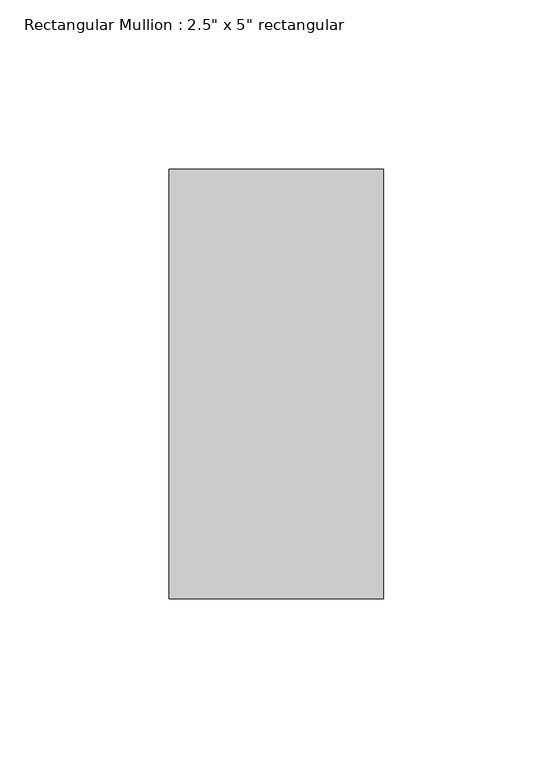
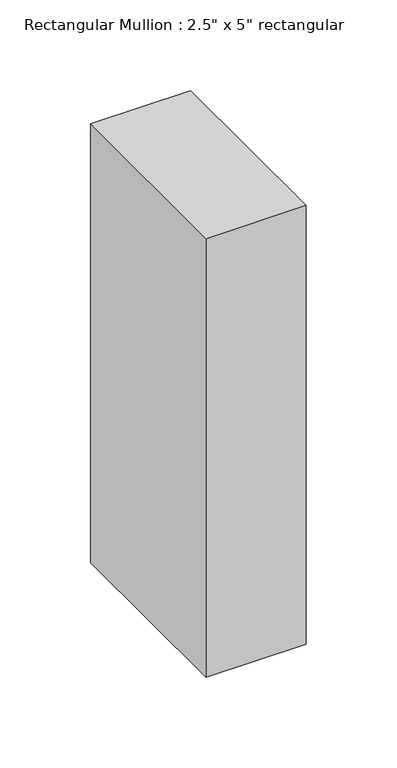
"""IFC4 building model written with IfcOpenShell, lengths in millimetres: member geometry."""

from ifc_helpers import new_model, si_unit, frame, origin, place, context, project, spatial, polyline, outline, extrude, source, transform, mapped, element, save


def member_044eafc8(model_context):
    return source(origin(), model_context, "Body", "SweptSolid", [
        extrude(outline(polyline([(0.0, 63.5), (0.0, -63.5), (-63.5, -63.5), (-63.5, 63.5), (0.0, 63.5)])), frame((0.0, 0.0, -294.64), z_axis=(0.0, 0.0, 1.0), x_axis=(1.0, 0.0, 0.0)), (0.0, 0.0, 1.0), 294.64),
    ])


if __name__ == "__main__":
    model = new_model("IFC4")
    model_context = context("Model", 3, world=origin())
    ifc_project = project(units=[si_unit("LENGTHUNIT", "METRE", prefix="MILLI")], contexts=[model_context])
    site = spatial("IfcSite", under=ifc_project)
    building = spatial("IfcBuilding", under=site)
    placement = place(None, origin())
    member_shape = member_044eafc8(model_context)
    element("IfcMember", 1, ObjectType="Rectangular Mullion : 2.5\" x 5\" rectangular", at=placement, inside=building, context=model_context, shape_type="MappedRepresentation", body=[
        mapped(member_shape, transform((0.0, 0.0, 0.0), x_axis=(1.0, 0.0, 0.0), y_axis=(0.0, 1.0, 0.0), z_axis=(0.0, 0.0, 1.0))),
    ])
    save(model, "model.ifc")

# Revit data of these elements
# Type "Rectangular Mullion : 2.5\" x 5\" rectangular"
#   built-in parameter 1007304 = 0.416667 (stored number, unit not read)
#   built-in parameter 1007301 = 0.104167 (stored number, unit not read)
#   built-in parameter 1007300 = 0.104167 (stored number, unit not read)
# Element 1 (IfcMember, "Rectangular Mullion : 2.5\" x 5\" rectangular")
#   Materials on its faces: "Aluminum"
# Materials
#   "Aluminum": class "Metal", colour RGB 247 247 247, transparency 0, Description = "Aluminum 6061", Cost = 0
